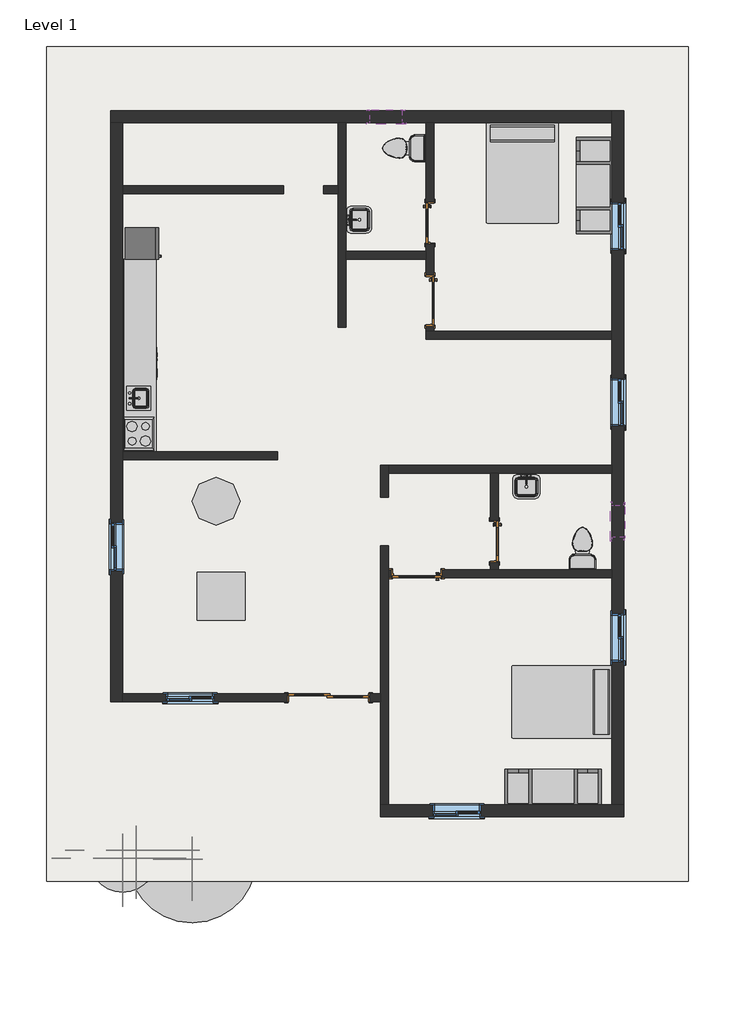
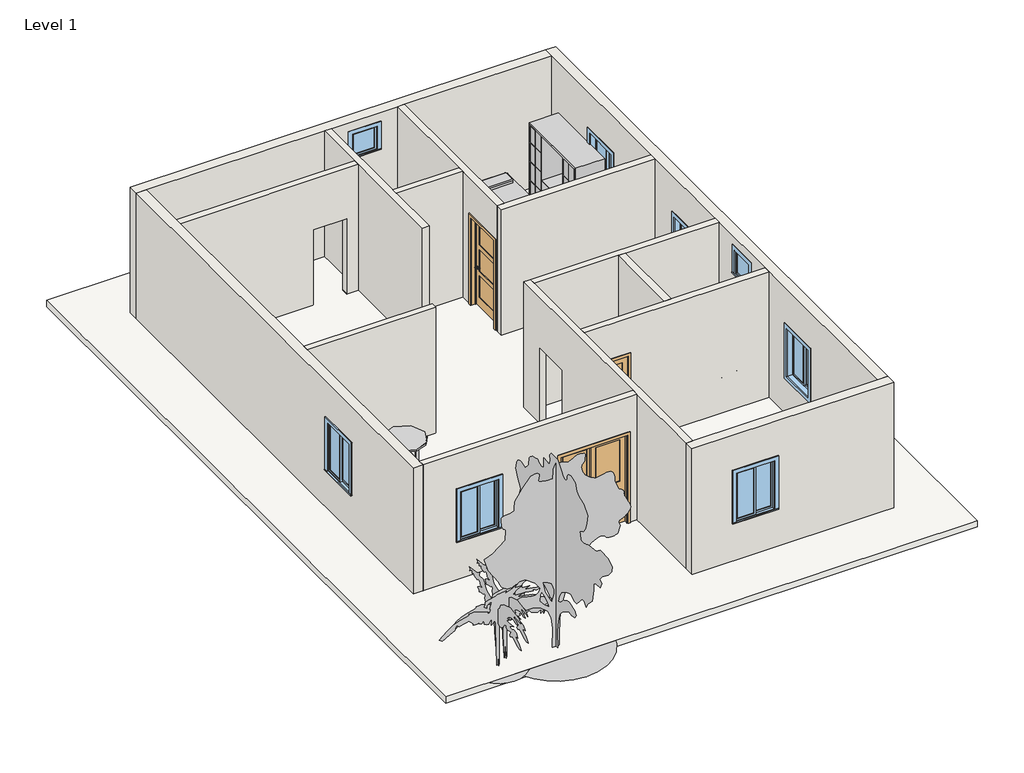
# One storey, incomplete: 15 walls, 8 windows, 7 furniture elements, 5 doors, 5 flow terminals, 4 proxies, 3 geographic elements, 1 slab.
"""IFC4 building model written with IfcOpenShell, lengths in millimetres."""

from ifc_helpers import new_model, si_unit, frame, origin, origin_with_axes, place, context, project, spatial, polyline, outline, extrude, faceted_brep, transform, mapped, element, save
from components import proxy_a6faaae8, proxy_45b28599, kitchenette_medium_kitchenette_medium_2_844211aa, proxy_c523a7b7, door_80d3ddc5, door_a1d926d7, door_7bbed545, door_8959c651, flow_terminal_871c2e40, flow_terminal_62a433f7, toilet_domestic_3d_toilet_domestic_3d_f7549cf7, toilet_domestic_3d_toilet_domestic_3d_183bbd19, furniture_0253826f, furniture_1317d646, furniture_cf0b6580, furniture_905aceb5, furniture_4d44e21c, rpc_tree_deciduous_japanese_cherry_15_e499737d, rpc_tree_tropical_australian_tree_furn_6_77f1a640, window_e25db5b6, window_99c3d43f, window_3ed046d9

model = new_model("IFC4")

# Units and contexts
model_context = context("Model", 3, world=origin())
ifc_project = project(units=[si_unit("LENGTHUNIT", "METRE", prefix="MILLI")], contexts=[model_context])

# Site, building, storey
site = spatial("IfcSite", under=ifc_project)
building = spatial("IfcBuilding", under=site)
storey = spatial("IfcBuildingStorey", under=building, Name="Level 1", Elevation=0.0)

# Proxies
placement = place(None, origin())
proxy_shape = proxy_a6faaae8(model_context)
element("IfcBuildingElementProxy", 1, Name="Cook Top-4 Unit2 : 22\" x 20\"", ObjectType="Cook Top-4 Unit2 : 22\" x 20\"", at=placement, inside=storey, context=model_context, shape_type="MappedRepresentation", body=[
    mapped(proxy_shape, transform((-13786.8447707, 5135.0679528, 0.0), x_axis=(0.0, 1.0000000000000002, 0.0), y_axis=(-1.0000000000000002, 0.0, 0.0), z_axis=(0.0, 0.0, 1.0))),
])
proxy_2_shape = proxy_45b28599(model_context)
element("IfcBuildingElementProxy", 2, Name="Dishwasher : 24\" x 24\" x 34\"", ObjectType="Dishwasher : 24\" x 24\" x 34\"", at=placement, inside=storey, context=model_context, shape_type="MappedRepresentation", body=[
    mapped(proxy_2_shape, transform((-13494.995206, 6086.2504843, 0.0), x_axis=(0.0, 1.0000000000000002, 0.0), y_axis=(-1.0000000000000002, 0.0, 0.0), z_axis=(0.0, 0.0, 1.0))),
])
kitchenette_medium_kitchenette_medium_2_shape = kitchenette_medium_kitchenette_medium_2_844211aa(model_context)
element("IfcBuildingElementProxy", 3, Name="Kitchenette - Medium : Kitchenette - Medium 2", ObjectType="Kitchenette - Medium : Kitchenette - Medium 2", at=placement, inside=storey, context=model_context, shape_type="MappedRepresentation", body=[
    mapped(kitchenette_medium_kitchenette_medium_2_shape, transform((-14091.6447707, 5459.2302479, 0.0), x_axis=(0.0, 1.0000000000000002, 0.0), y_axis=(-1.0000000000000002, 0.0, 0.0), z_axis=(0.0, 0.0, 1.0))),
])
proxy_3_shape = proxy_c523a7b7(model_context)
element("IfcBuildingElementProxy", 4, Name="Refrigerator : 24\" x 25\" LH", ObjectType="Refrigerator : 24\" x 25\" LH", at=placement, inside=storey, context=model_context, shape_type="MappedRepresentation", body=[
    mapped(proxy_3_shape, transform((-13741.1957993, 8748.2179528, 0.0), x_axis=(0.0, 1.0000000000000002, 0.0), y_axis=(-1.0000000000000002, 0.0, 0.0), z_axis=(0.0, 0.0, 1.0))),
])

# Doors
door_shape = door_80d3ddc5(model_context)
element("IfcDoor", 5, ObjectType="Door-Interior-Double-Sliding-2_Panel-Wood : 60\" x 84\"", at=placement, inside=storey, context=model_context, shape_type="MappedRepresentation", body=[
    mapped(door_shape, transform((-10180.0447707, 121.7429528, 0.0), x_axis=(1.0, 0.0, 0.0), y_axis=(0.0, 1.0, 0.0), z_axis=(0.0, 0.0, 1.0))),
])
door_2_shape = door_a1d926d7(model_context)
element("IfcDoor", 6, ObjectType="Door-Interior-Single-1_Panel-Wood : 30\" x 80\"", at=placement, inside=storey, context=model_context, shape_type="MappedRepresentation", body=[
    mapped(door_2_shape, transform((-7027.2697707, 3090.3679528, 0.0), x_axis=(0.0, -1.0, 0.0), y_axis=(1.0, 0.0, 0.0), z_axis=(0.0, 0.0, 1.0))),
])
door_3_shape = door_7bbed545(model_context)
element("IfcDoor", 7, ObjectType="Door-Interior-Single-1_Panel-Wood : 30\" x 80\"", at=placement, inside=storey, context=model_context, shape_type="MappedRepresentation", body=[
    mapped(door_3_shape, transform((-8252.8197707, 9135.5679528, 0.0), x_axis=(0.0, -1.0, 0.0), y_axis=(1.0, 0.0, 0.0), z_axis=(0.0, 0.0, 1.0))),
])
door_4_shape = door_8959c651(model_context)
element("IfcDoor", 8, ObjectType="Door-Interior-Single-3_Panel_Vert-Wood : 36\" x 84\"", at=placement, inside=storey, context=model_context, shape_type="MappedRepresentation", body=[
    mapped(door_4_shape, transform((-8503.6447707, 2477.5929528, 0.0), x_axis=(-1.0, 0.0, 0.0), y_axis=(0.0, -1.0, 0.0), z_axis=(0.0, 0.0, 1.0))),
])
element("IfcDoor", 9, ObjectType="Door-Interior-Single-3_Panel_Vert-Wood : 36\" x 84\"", at=placement, inside=storey, context=model_context, shape_type="MappedRepresentation", body=[
    mapped(door_4_shape, transform((-8246.4697707, 7662.3679528, 0.0), x_axis=(0.0, -1.0, 0.0), y_axis=(1.0, 0.0, 0.0), z_axis=(0.0, 0.0, 1.0))),
])

# Flow terminals
flow_terminal_shape = flow_terminal_871c2e40(model_context)
element("IfcFlowTerminal", 10, ObjectType="Sink Kitchen-Island : 18\" x 18\"", at=placement, inside=storey, context=model_context, shape_type="MappedRepresentation", body=[
    mapped(flow_terminal_shape, transform((-13784.4993696, 5792.4787122, -14.4), x_axis=(0.0, 1.0000000000000002, 0.0), y_axis=(-1.0000000000000002, 0.0, 0.0), z_axis=(0.0, 0.0, 1.0))),
])
flow_terminal_2_shape = flow_terminal_62a433f7(model_context)
element("IfcFlowTerminal", 11, ObjectType="Sink Vanity-Square : 20\" x 18\"", at=placement, inside=storey, context=model_context, shape_type="MappedRepresentation", body=[
    mapped(flow_terminal_2_shape, transform((-9644.2993696, 9183.3787122, 0.0), x_axis=(0.0, 1.0000000000000002, 0.0), y_axis=(-1.0000000000000002, 0.0, 0.0), z_axis=(0.0, 0.0, 1.0))),
])
element("IfcFlowTerminal", 12, ObjectType="Sink Vanity-Square : 20\" x 18\"", at=placement, inside=storey, context=model_context, shape_type="MappedRepresentation", body=[
    mapped(flow_terminal_2_shape, transform((-6436.5340113, 4180.2225517, 0.0), x_axis=(1.0000000000000007, 0.0, 0.0), y_axis=(0.0, 1.0000000000000007, 0.0), z_axis=(0.0, 0.0, 1.0))),
])
toilet_domestic_3d_toilet_domestic_3d_shape = toilet_domestic_3d_toilet_domestic_3d_f7549cf7(model_context)
toilet_domestic_3d_toilet_domestic_3d_2_shape = toilet_domestic_3d_toilet_domestic_3d_183bbd19(model_context)
element("IfcFlowTerminal", 13, ObjectType="Toilet-Domestic-3D : Toilet-Domestic-3D", at=placement, inside=storey, context=model_context, shape_type="MappedRepresentation", body=[
    mapped(toilet_domestic_3d_toilet_domestic_3d_shape, transform((-8845.9407981, 10557.9679528, 0.0), x_axis=(0.0, -1.0000000000000004, 0.0), y_axis=(1.0000000000000004, 0.0, 0.0), z_axis=(0.0, 0.0, 1.0))),
    mapped(toilet_domestic_3d_toilet_domestic_3d_2_shape, transform((-8845.9407981, 10557.9679528, 0.0), x_axis=(0.0, -1.0000000000000004, 0.0), y_axis=(1.0000000000000004, 0.0, 0.0), z_axis=(0.0, 0.0, 1.0))),
])
element("IfcFlowTerminal", 14, ObjectType="Toilet-Domestic-3D : Toilet-Domestic-3D", at=placement, inside=storey, context=model_context, shape_type="MappedRepresentation", body=[
    mapped(toilet_domestic_3d_toilet_domestic_3d_shape, transform((-5354.0447707, 3051.6639802, 0.0), x_axis=(-1.0000000000000004, 0.0, 0.0), y_axis=(0.0, -1.0000000000000004, 0.0), z_axis=(0.0, 0.0, 1.0))),
    mapped(toilet_domestic_3d_toilet_domestic_3d_2_shape, transform((-5354.0447707, 3051.6639802, 0.0), x_axis=(-1.0000000000000004, 0.0, 0.0), y_axis=(0.0, -1.0000000000000004, 0.0), z_axis=(0.0, 0.0, 1.0))),
])

# Furniture
furniture_shape = furniture_0253826f(model_context)
element("IfcFurniture", 15, ObjectType="Bed-Standard : Double 54\" x 75\"", at=placement, inside=storey, context=model_context, shape_type="MappedRepresentation", body=[
    mapped(furniture_shape, transform((-6768.5332953, 10133.6630348, 0.0), x_axis=(1.0, 0.0, 0.0), y_axis=(0.0, 1.0, 0.0), z_axis=(0.0, 0.0, 1.0))),
])
element("IfcFurniture", 16, ObjectType="Bed-Standard : Double 54\" x 75\"", at=placement, inside=storey, context=model_context, shape_type="MappedRepresentation", body=[
    mapped(furniture_shape, transform((-5702.1496888, 313.8564774, 0.0), x_axis=(0.0, -1.0, 0.0), y_axis=(1.0, 0.0, 0.0), z_axis=(0.0, 0.0, 1.0))),
])
furniture_2_shape = furniture_1317d646(model_context)
element("IfcFurniture", 17, ObjectType="Counter Top w Sink Hole : 24\" Depth", at=placement, inside=storey, context=model_context, shape_type="MappedRepresentation", body=[
    mapped(furniture_2_shape, transform((-14091.6447707, 5992.6302479, -14.4), x_axis=(0.0, 1.0000000000000002, 0.0), y_axis=(-1.0000000000000002, 0.0, 0.0), z_axis=(0.0, 0.0, 1.0))),
])
furniture_3_shape = furniture_cf0b6580(model_context)
element("IfcFurniture", 18, ObjectType="Entertainment Center : 72\" x 72\" x 24\"", at=placement, inside=storey, context=model_context, shape_type="MappedRepresentation", body=[
    mapped(furniture_3_shape, transform((-5912.8447707, -2015.0320472, 0.0), x_axis=(-1.0, 0.0, 0.0), y_axis=(0.0, -1.0, 0.0), z_axis=(0.0, 0.0, 1.0))),
])
element("IfcFurniture", 19, ObjectType="Entertainment Center : 72\" x 72\" x 24\"", at=placement, inside=storey, context=model_context, shape_type="MappedRepresentation", body=[
    mapped(furniture_3_shape, transform((-4693.6447707, 9846.7679528, 0.0), x_axis=(0.0, -1.0000000000000002, 0.0), y_axis=(1.0000000000000002, 0.0, 0.0), z_axis=(0.0, 0.0, 1.0))),
])
furniture_4_shape = furniture_905aceb5(model_context)
element("IfcFurniture", 20, ObjectType="Table-Dining Round w Chairs : 36\" Diameter", at=placement, inside=storey, context=model_context, shape_type="MappedRepresentation", body=[
    mapped(furniture_4_shape, transform((-12417.326738, 4037.2466413, 0.0), x_axis=(1.0, 0.0, 0.0), y_axis=(0.0, 1.0, 0.0), z_axis=(0.0, 0.0, 1.0))),
])
furniture_5_shape = furniture_4d44e21c(model_context)
element("IfcFurniture", 21, ObjectType="Table-Rectangular : 36\" x 36\"", at=placement, inside=storey, context=model_context, shape_type="MappedRepresentation", body=[
    mapped(furniture_5_shape, transform((-12224.7447707, 2048.9679528, 0.0), x_axis=(0.0, 1.0000000000000002, 0.0), y_axis=(-1.0000000000000002, 0.0, 0.0), z_axis=(0.0, 0.0, 1.0))),
])

# Geographic elements
rpc_tree_deciduous_japanese_cherry_15_shape = rpc_tree_deciduous_japanese_cherry_15_e499737d(model_context)
element("IfcGeographicElement", 22, ObjectType="RPC Tree - Deciduous : Japanese Cherry - 15'", at=placement, inside=storey, context=model_context, shape_type="MappedRepresentation", body=[
    mapped(rpc_tree_deciduous_japanese_cherry_15_shape, transform((-12770.8447707, -2942.1320472, 0.0), x_axis=(1.0, 0.0, 0.0), y_axis=(0.0, 1.0, 0.0), z_axis=(0.0, 0.0, 1.0))),
])
rpc_tree_tropical_australian_tree_furn_6_shape = rpc_tree_tropical_australian_tree_furn_6_77f1a640(model_context)
element("IfcGeographicElement", 23, ObjectType="RPC Tree - Tropical : Australian Tree Furn - 6'", at=placement, inside=storey, context=model_context, shape_type="MappedRepresentation", body=[
    mapped(rpc_tree_tropical_australian_tree_furn_6_shape, transform((-13837.6447707, -2777.0320472, 0.0), x_axis=(1.0, 0.0, 0.0), y_axis=(0.0, 1.0, 0.0), z_axis=(0.0, 0.0, 1.0))),
])
element("IfcGeographicElement", 24, ObjectType="RPC Tree - Tropical : Australian Tree Furn - 6'", at=placement, inside=storey, context=model_context, shape_type="MappedRepresentation", body=[
    mapped(rpc_tree_tropical_australian_tree_furn_6_shape, transform((-14091.6447707, -2929.4320472, 0.0), x_axis=(1.0, 0.0, 0.0), y_axis=(0.0, 1.0, 0.0), z_axis=(0.0, 0.0, 1.0))),
])

# Slab
element("IfcSlab", 25, ObjectType="Generic - 6\" 2", at=placement, inside=storey, context=model_context, shape_type="SweptSolid", body=[
    extrude(outline(polyline([(-3347.4447707, 12488.3679528), (-3347.4447707, -3361.2320472), (-15539.4447707, -3361.2320472), (-15539.4447707, 12488.3679528), (-3347.4447707, 12488.3679528)])), frame((0.0, 0.0, -152.4), z_axis=(0.0, 0.0, 1.0), x_axis=(1.0, 0.0, 0.0)), (0.0, 0.0, 1.0), 152.4),
])

# Walls
element("IfcWall", 26, ObjectType="Generic - 6\"", at=placement, inside=storey, context=model_context, shape_type="Brep", body=[
    faceted_brep([(-4795.2447707, 7078.1679528, 0.0), (-8173.4447707, 7078.1679528, 0.0), (-8325.8447707, 7078.1679528, 0.0), (-8325.8447707, 7078.1679528, 3048.0), (-8173.4447707, 7078.1679528, 3048.0), (-4795.2447707, 7078.1679528, 3048.0), (-4795.2447707, 6925.7679528, 0.0), (-4795.2447707, 6925.7679528, 3048.0), (-8325.8447707, 6925.7679528, 3048.0), (-8325.8447707, 6925.7679528, 0.0)], [[[0, 1, 2, 3, 4, 5]], [[6, 7, 8, 9]], [[2, 1, 0, 6, 9]], [[5, 4, 3, 8, 7]], [[0, 5, 7, 6]], [[3, 2, 9, 8]]]),
])
element("IfcWall", 27, ObjectType="Generic - 6\"", at=placement, inside=storey, context=model_context, shape_type="Brep", body=[
    faceted_brep([(-8325.8447707, 7078.1679528, 3048.0), (-8325.8447707, 8449.7679528, 3048.0), (-8325.8447707, 8602.1679528, 3048.0), (-8325.8447707, 11040.5679528, 3048.0), (-8325.8447707, 11040.5679528, 0.0), (-8325.8447707, 9541.9679528, 0.0), (-8325.8447707, 9541.9679528, 2057.4), (-8325.8447707, 8729.1679528, 2057.4), (-8325.8447707, 8729.1679528, 0.0), (-8325.8447707, 8602.1679528, 0.0), (-8325.8447707, 8449.7679528, 0.0), (-8325.8447707, 8144.9679528, 0.0), (-8325.8447707, 8144.9679528, 2159.0), (-8325.8447707, 7179.7679528, 2159.0), (-8325.8447707, 7179.7679528, 0.0), (-8325.8447707, 7078.1679528, 0.0), (-8173.4447707, 11040.5679528, 3048.0), (-8173.4447707, 7078.1679528, 3048.0), (-8173.4447707, 7078.1679528, 0.0), (-8173.4447707, 7179.7679528, 0.0), (-8173.4447707, 7179.7679528, 2159.0), (-8173.4447707, 8144.9679528, 2159.0), (-8173.4447707, 8144.9679528, 0.0), (-8173.4447707, 8729.1679528, 0.0), (-8173.4447707, 8729.1679528, 2057.4), (-8173.4447707, 9541.9679528, 2057.4), (-8173.4447707, 9541.9679528, 0.0), (-8173.4447707, 11040.5679528, 0.0)], [[[0, 1, 2, 3, 4, 5, 6, 7, 8, 9, 10, 11, 12, 13, 14, 15]], [[16, 17, 18, 19, 20, 21, 22, 23, 24, 25, 26, 27]], [[4, 27, 26, 5]], [[18, 15, 14, 19]], [[22, 11, 10, 9, 8, 23]], [[3, 2, 1, 0, 17, 16]], [[4, 3, 16, 27]], [[0, 15, 18, 17]], [[13, 20, 19, 14]], [[20, 13, 12, 21]], [[21, 12, 11, 22]], [[7, 24, 23, 8]], [[24, 7, 6, 25]], [[25, 6, 5, 26]]]),
])
element("IfcWall", 28, ObjectType="Generic - 6\"", at=placement, inside=storey, context=model_context, shape_type="SweptSolid", body=[
    extrude(outline(polyline([(-9849.8447707, 8602.1679528), (-8325.8447707, 8602.1679528), (-8325.8447707, 8449.7679528), (-9849.8447707, 8449.7679528), (-9849.8447707, 8602.1679528)])), origin_with_axes(), (0.0, 0.0, 1.0), 3048.0),
])
element("IfcWall", 29, ObjectType="Generic - 6\"", at=placement, inside=storey, context=model_context, shape_type="Brep", body=[
    faceted_brep([(-10002.2447707, 11040.5679528, 0.0), (-10002.2447707, 9846.7679528, 0.0), (-10002.2447707, 9694.3679528, 0.0), (-10002.2447707, 7154.3679528, 0.0), (-10002.2447707, 7154.3679528, 3048.0), (-10002.2447707, 9694.3679528, 3048.0), (-10002.2447707, 9846.7679528, 3048.0), (-10002.2447707, 11040.5679528, 3048.0), (-9849.8447707, 11040.5679528, 0.0), (-9849.8447707, 11040.5679528, 3048.0), (-9849.8447707, 8602.1679528, 3048.0), (-9849.8447707, 8449.7679528, 3048.0), (-9849.8447707, 7154.3679528, 3048.0), (-9849.8447707, 7154.3679528, 0.0), (-9849.8447707, 8449.7679528, 0.0), (-9849.8447707, 8602.1679528, 0.0)], [[[0, 1, 2, 3, 4, 5, 6, 7]], [[8, 9, 10, 11, 12, 13, 14, 15]], [[3, 2, 1, 0, 8, 15, 14, 13]], [[4, 3, 13, 12]], [[7, 6, 5, 4, 12, 11, 10, 9]], [[0, 7, 9, 8]]]),
])
element("IfcWall", 30, ObjectType="Generic - 6\"", at=placement, inside=storey, context=model_context, shape_type="SweptSolid", body=[
    extrude(outline(polyline([(0.0, -10002.2447707), (3048.0, -10002.2447707), (3048.0, -14091.6447707), (0.0, -14091.6447707), (0.0, -11037.2947707), (12.7, -11037.2947707), (1828.8, -11037.2947707), (1828.8, -10275.2947707), (12.7, -10275.2947707), (0.0, -10275.2947707), (0.0, -10002.2447707)])), frame((0.0, 9694.3679528, 0.0), z_axis=(0.0, 1.0, 0.0), x_axis=(0.0, 0.0, 1.0)), (0.0, 0.0, 1.0), 152.4),
])
element("IfcWall", 31, ObjectType="Generic - 6\"", at=placement, inside=storey, context=model_context, shape_type="SweptSolid", body=[
    extrude(outline(polyline([(3048.0, -9189.4447707), (3048.0, -14091.6447707), (0.0, -14091.6447707), (0.0, -10967.4447707), (2159.0, -10967.4447707), (2159.0, -9392.6447707), (0.0, -9392.6447707), (0.0, -9189.4447707), (3048.0, -9189.4447707)]), holes=[polyline([(2133.6, -13266.1447707), (2133.6, -12351.7447707), (914.4, -12351.7447707), (914.4, -13266.1447707), (2133.6, -13266.1447707)])]), frame((0.0, 42.3679528, 0.0), z_axis=(0.0, 1.0, 0.0), x_axis=(0.0, 0.0, 1.0)), (0.0, 0.0, 1.0), 152.4),
])
element("IfcWall", 32, ObjectType="Generic - 6\"", at=placement, inside=storey, context=model_context, shape_type="Brep", body=[
    faceted_brep([(-9189.4447707, 4538.1679528, 0.0), (-9189.4447707, 3925.3929528, 0.0), (-9189.4447707, 3925.3929528, 1828.8), (-9189.4447707, 3010.9929528, 1828.8), (-9189.4447707, 3010.9929528, 0.0), (-9189.4447707, 194.7679528, 0.0), (-9189.4447707, 42.3679528, 0.0), (-9189.4447707, -1913.4320472, 0.0), (-9189.4447707, -1913.4320472, 3048.0), (-9189.4447707, 42.3679528, 3048.0), (-9189.4447707, 194.7679528, 3048.0), (-9189.4447707, 4538.1679528, 3048.0), (-9037.0447707, 4538.1679528, 0.0), (-9037.0447707, 4538.1679528, 3048.0), (-9037.0447707, 4385.7679528, 3048.0), (-9037.0447707, 2556.9679528, 3048.0), (-9037.0447707, 2404.5679528, 3048.0), (-9037.0447707, -1913.4320472, 3048.0), (-9037.0447707, -1913.4320472, 0.0), (-9037.0447707, 2404.5679528, 0.0), (-9037.0447707, 2556.9679528, 0.0), (-9037.0447707, 3010.9929528, 0.0), (-9037.0447707, 3010.9929528, 1828.8), (-9037.0447707, 3925.3929528, 1828.8), (-9037.0447707, 3925.3929528, 0.0), (-9037.0447707, 4385.7679528, 0.0)], [[[0, 1, 2, 3, 4, 5, 6, 7, 8, 9, 10, 11]], [[12, 13, 14, 15, 16, 17, 18, 19, 20, 21, 22, 23, 24, 25]], [[0, 11, 13, 12]], [[8, 7, 18, 17]], [[1, 0, 12, 25, 24]], [[11, 10, 9, 8, 17, 16, 15, 14, 13]], [[2, 1, 24, 23]], [[3, 2, 23, 22]], [[4, 3, 22, 21]], [[7, 6, 5, 4, 21, 20, 19, 18]]]),
])
element("IfcWall", 33, ObjectType="Generic - 6\"", at=placement, inside=storey, context=model_context, shape_type="Brep", body=[
    faceted_brep([(-9037.0447707, 2556.9679528, 3048.0), (-7106.6447707, 2556.9679528, 3048.0), (-6954.2447707, 2556.9679528, 3048.0), (-4795.2447707, 2556.9679528, 3048.0), (-4795.2447707, 2556.9679528, 0.0), (-6954.2447707, 2556.9679528, 0.0), (-7106.6447707, 2556.9679528, 0.0), (-8021.0447707, 2556.9679528, 0.0), (-8021.0447707, 2556.9679528, 2159.0), (-8986.2447707, 2556.9679528, 2159.0), (-8986.2447707, 2556.9679528, 0.0), (-9037.0447707, 2556.9679528, 0.0), (-4795.2447707, 2404.5679528, 3048.0), (-9037.0447707, 2404.5679528, 3048.0), (-9037.0447707, 2404.5679528, 0.0), (-8986.2447707, 2404.5679528, 0.0), (-8986.2447707, 2404.5679528, 2159.0), (-8021.0447707, 2404.5679528, 2159.0), (-8021.0447707, 2404.5679528, 0.0), (-4795.2447707, 2404.5679528, 0.0)], [[[0, 1, 2, 3, 4, 5, 6, 7, 8, 9, 10, 11]], [[12, 13, 14, 15, 16, 17, 18, 19]], [[4, 19, 18, 7, 6, 5]], [[14, 11, 10, 15]], [[3, 2, 1, 0, 13, 12]], [[4, 3, 12, 19]], [[0, 11, 14, 13]], [[9, 16, 15, 10]], [[16, 9, 8, 17]], [[17, 8, 7, 18]]]),
])
element("IfcWall", 34, ObjectType="Generic - 6\"", at=placement, inside=storey, context=model_context, shape_type="Brep", body=[
    faceted_brep([(-4795.2447707, 4538.1679528, 0.0), (-9037.0447707, 4538.1679528, 0.0), (-9037.0447707, 4538.1679528, 3048.0), (-4795.2447707, 4538.1679528, 3048.0), (-4795.2447707, 4385.7679528, 0.0), (-4795.2447707, 4385.7679528, 3048.0), (-6954.2447707, 4385.7679528, 3048.0), (-7106.6447707, 4385.7679528, 3048.0), (-9037.0447707, 4385.7679528, 3048.0), (-9037.0447707, 4385.7679528, 0.0), (-7106.6447707, 4385.7679528, 0.0), (-6954.2447707, 4385.7679528, 0.0)], [[[0, 1, 2, 3]], [[4, 5, 6, 7, 8, 9, 10, 11]], [[1, 0, 4, 11, 10, 9]], [[3, 2, 8, 7, 6, 5]], [[0, 3, 5, 4]], [[2, 1, 9, 8]]]),
])
element("IfcWall", 35, ObjectType="Generic - 6\"", at=placement, inside=storey, context=model_context, shape_type="SweptSolid", body=[
    extrude(outline(polyline([(2556.9679528, 3048.0), (4385.7679528, 3048.0), (4385.7679528, 0.0), (3496.7679528, 0.0), (3496.7679528, 2057.4), (2683.9679528, 2057.4), (2683.9679528, 0.0), (2556.9679528, 0.0), (2556.9679528, 3048.0)])), frame((-7106.6447707, 0.0, 0.0), z_axis=(1.0, 0.0, 0.0), x_axis=(0.0, 1.0, 0.0)), (0.0, 0.0, 1.0), 152.4),
])
element("IfcWall", 36, ObjectType="Generic - 6\"", at=placement, inside=storey, context=model_context, shape_type="SweptSolid", body=[
    extrude(outline(polyline([(-14091.6447707, 4792.1679528), (-11145.2447707, 4792.1679528), (-11145.2447707, 4639.7679528), (-14091.6447707, 4639.7679528), (-14091.6447707, 4792.1679528)])), origin_with_axes(), (0.0, 0.0, 1.0), 3048.0),
])
element("IfcWall", 37, ObjectType="Generic - 9\" 2", at=placement, inside=storey, context=model_context, shape_type="Brep", body=[
    faceted_brep([(-14320.2447707, 11040.5679528, 0.0), (-14091.6447707, 11040.5679528, 0.0), (-10002.2447707, 11040.5679528, 0.0), (-9849.8447707, 11040.5679528, 0.0), (-8325.8447707, 11040.5679528, 0.0), (-8173.4447707, 11040.5679528, 0.0), (-4795.2447707, 11040.5679528, 0.0), (-4795.2447707, 11040.5679528, 3048.0), (-8173.4447707, 11040.5679528, 3048.0), (-8325.8447707, 11040.5679528, 3048.0), (-9849.8447707, 11040.5679528, 3048.0), (-10002.2447707, 11040.5679528, 3048.0), (-14091.6447707, 11040.5679528, 3048.0), (-14320.2447707, 11040.5679528, 3048.0), (-9392.6447707, 11040.5679528, 2768.6), (-8783.0447707, 11040.5679528, 2768.6), (-8783.0447707, 11040.5679528, 2159.0), (-9392.6447707, 11040.5679528, 2159.0), (-14320.2447707, 11269.1679528, 0.0), (-14320.2447707, 11269.1679528, 3048.0), (-4795.2447707, 11269.1679528, 3048.0), (-4795.2447707, 11269.1679528, 0.0), (-9392.6447707, 11269.1679528, 2768.6), (-9392.6447707, 11269.1679528, 2159.0), (-8783.0447707, 11269.1679528, 2159.0), (-8783.0447707, 11269.1679528, 2768.6)], [[[0, 1, 2, 3, 4, 5, 6, 7, 8, 9, 10, 11, 12, 13], [14, 15, 16, 17]], [[18, 19, 20, 21], [22, 23, 24, 25]], [[6, 5, 4, 3, 2, 1, 0, 18, 21]], [[13, 12, 11, 10, 9, 8, 7, 20, 19]], [[0, 13, 19, 18]], [[7, 6, 21, 20]], [[23, 22, 14, 17]], [[24, 23, 17, 16]], [[25, 24, 16, 15]], [[22, 25, 15, 14]]]),
])
element("IfcWall", 38, ObjectType="Generic - 9\" 2", at=placement, inside=storey, context=model_context, shape_type="Brep", body=[
    faceted_brep([(-14091.6447707, 42.3679528, 0.0), (-14091.6447707, 194.7679528, 0.0), (-14091.6447707, 4639.7679528, 0.0), (-14091.6447707, 4792.1679528, 0.0), (-14091.6447707, 9694.3679528, 0.0), (-14091.6447707, 9846.7679528, 0.0), (-14091.6447707, 11040.5679528, 0.0), (-14091.6447707, 11040.5679528, 3048.0), (-14091.6447707, 9846.7679528, 3048.0), (-14091.6447707, 9694.3679528, 3048.0), (-14091.6447707, 4792.1679528, 3048.0), (-14091.6447707, 4639.7679528, 3048.0), (-14091.6447707, 194.7679528, 3048.0), (-14091.6447707, 42.3679528, 3048.0), (-14091.6447707, 3445.9679528, 2133.6), (-14091.6447707, 3445.9679528, 914.4), (-14091.6447707, 2531.5679528, 914.4), (-14091.6447707, 2531.5679528, 2133.6), (-14320.2447707, 42.3679528, 0.0), (-14320.2447707, 42.3679528, 3048.0), (-14320.2447707, 11040.5679528, 3048.0), (-14320.2447707, 11040.5679528, 0.0), (-14320.2447707, 3445.9679528, 2133.6), (-14320.2447707, 2531.5679528, 2133.6), (-14320.2447707, 2531.5679528, 914.4), (-14320.2447707, 3445.9679528, 914.4)], [[[0, 1, 2, 3, 4, 5, 6, 7, 8, 9, 10, 11, 12, 13], [14, 15, 16, 17]], [[18, 19, 20, 21], [22, 23, 24, 25]], [[6, 5, 4, 3, 2, 1, 0, 18, 21]], [[13, 12, 11, 10, 9, 8, 7, 20, 19]], [[7, 6, 21, 20]], [[15, 14, 22, 25]], [[16, 15, 25, 24]], [[17, 16, 24, 23]], [[14, 17, 23, 22]], [[0, 13, 19, 18]]]),
])
element("IfcWall", 39, ObjectType="Generic - 9\" 2", at=placement, inside=storey, context=model_context, shape_type="Brep", body=[
    faceted_brep([(-4566.6447707, -1913.4320472, 0.0), (-4795.2447707, -1913.4320472, 0.0), (-9037.0447707, -1913.4320472, 0.0), (-9189.4447707, -1913.4320472, 0.0), (-9189.4447707, -1913.4320472, 3048.0), (-9037.0447707, -1913.4320472, 3048.0), (-4795.2447707, -1913.4320472, 3048.0), (-4566.6447707, -1913.4320472, 3048.0), (-8198.8447707, -1913.4320472, 2133.6), (-8198.8447707, -1913.4320472, 914.4), (-7284.4447707, -1913.4320472, 914.4), (-7284.4447707, -1913.4320472, 2133.6), (-4566.6447707, -2142.0320472, 0.0), (-4566.6447707, -2142.0320472, 3048.0), (-9189.4447707, -2142.0320472, 3048.0), (-9189.4447707, -2142.0320472, 0.0), (-8198.8447707, -2142.0320472, 2133.6), (-7284.4447707, -2142.0320472, 2133.6), (-7284.4447707, -2142.0320472, 914.4), (-8198.8447707, -2142.0320472, 914.4)], [[[0, 1, 2, 3, 4, 5, 6, 7], [8, 9, 10, 11]], [[12, 13, 14, 15], [16, 17, 18, 19]], [[3, 2, 1, 0, 12, 15]], [[7, 6, 5, 4, 14, 13]], [[0, 7, 13, 12]], [[4, 3, 15, 14]], [[9, 8, 16, 19]], [[10, 9, 19, 18]], [[11, 10, 18, 17]], [[8, 11, 17, 16]]]),
])
element("IfcWall", 40, ObjectType="Generic - 9\" 2", at=placement, inside=storey, context=model_context, shape_type="Brep", body=[
    faceted_brep([(-4795.2447707, 11269.1679528, 0.0), (-4795.2447707, 11040.5679528, 0.0), (-4795.2447707, 7078.1679528, 0.0), (-4795.2447707, 6925.7679528, 0.0), (-4795.2447707, 4538.1679528, 0.0), (-4795.2447707, 4385.7679528, 0.0), (-4795.2447707, 2556.9679528, 0.0), (-4795.2447707, 2404.5679528, 0.0), (-4795.2447707, -1913.4320472, 0.0), (-4795.2447707, -1913.4320472, 3048.0), (-4795.2447707, 2404.5679528, 3048.0), (-4795.2447707, 2556.9679528, 3048.0), (-4795.2447707, 4385.7679528, 3048.0), (-4795.2447707, 4538.1679528, 3048.0), (-4795.2447707, 6925.7679528, 3048.0), (-4795.2447707, 7078.1679528, 3048.0), (-4795.2447707, 11040.5679528, 3048.0), (-4795.2447707, 11269.1679528, 3048.0), (-4795.2447707, 5274.7679528, 2133.6), (-4795.2447707, 5274.7679528, 914.4), (-4795.2447707, 6189.1679528, 914.4), (-4795.2447707, 6189.1679528, 2133.6), (-4795.2447707, 8621.2179528, 2133.6), (-4795.2447707, 8621.2179528, 914.4), (-4795.2447707, 9535.6179528, 914.4), (-4795.2447707, 9535.6179528, 2133.6), (-4795.2447707, 804.3679528, 2133.6), (-4795.2447707, 804.3679528, 914.4), (-4795.2447707, 1718.7679528, 914.4), (-4795.2447707, 1718.7679528, 2133.6), (-4795.2447707, 3776.1679528, 2768.6), (-4795.2447707, 3166.5679528, 2768.6), (-4795.2447707, 3166.5679528, 2159.0), (-4795.2447707, 3776.1679528, 2159.0), (-4566.6447707, 11269.1679528, 0.0), (-4566.6447707, 11269.1679528, 3048.0), (-4566.6447707, -1913.4320472, 3048.0), (-4566.6447707, -1913.4320472, 0.0), (-4566.6447707, 5274.7679528, 2133.6), (-4566.6447707, 6189.1679528, 2133.6), (-4566.6447707, 6189.1679528, 914.4), (-4566.6447707, 5274.7679528, 914.4), (-4566.6447707, 8621.2179528, 2133.6), (-4566.6447707, 9535.6179528, 2133.6), (-4566.6447707, 9535.6179528, 914.4), (-4566.6447707, 8621.2179528, 914.4), (-4566.6447707, 804.3679528, 2133.6), (-4566.6447707, 1718.7679528, 2133.6), (-4566.6447707, 1718.7679528, 914.4), (-4566.6447707, 804.3679528, 914.4), (-4566.6447707, 3776.1679528, 2768.6), (-4566.6447707, 3776.1679528, 2159.0), (-4566.6447707, 3166.5679528, 2159.0), (-4566.6447707, 3166.5679528, 2768.6)], [[[0, 1, 2, 3, 4, 5, 6, 7, 8, 9, 10, 11, 12, 13, 14, 15, 16, 17], [18, 19, 20, 21], [22, 23, 24, 25], [26, 27, 28, 29], [30, 31, 32, 33]], [[34, 35, 36, 37], [38, 39, 40, 41], [42, 43, 44, 45], [46, 47, 48, 49], [50, 51, 52, 53]], [[8, 7, 6, 5, 4, 3, 2, 1, 0, 34, 37]], [[17, 16, 15, 14, 13, 12, 11, 10, 9, 36, 35]], [[0, 17, 35, 34]], [[9, 8, 37, 36]], [[19, 18, 38, 41]], [[20, 19, 41, 40]], [[21, 20, 40, 39]], [[18, 21, 39, 38]], [[23, 22, 42, 45]], [[24, 23, 45, 44]], [[25, 24, 44, 43]], [[22, 25, 43, 42]], [[27, 26, 46, 49]], [[28, 27, 49, 48]], [[29, 28, 48, 47]], [[26, 29, 47, 46]], [[51, 50, 30, 33]], [[52, 51, 33, 32]], [[53, 52, 32, 31]], [[50, 53, 31, 30]]]),
])

# Windows
window_shape = window_e25db5b6(model_context)
element("IfcWindow", 41, ObjectType="Slider with Trim : 36\" x 48\"", at=placement, inside=storey, context=model_context, shape_type="MappedRepresentation", body=[
    mapped(window_shape, transform((-14205.9447707, 2988.7679528, 0.0), x_axis=(0.0, 1.0, 0.0), y_axis=(-1.0, 0.0, 0.0), z_axis=(0.0, 0.0, 1.0))),
])
element("IfcWindow", 42, ObjectType="Slider with Trim : 36\" x 48\"", at=placement, inside=storey, context=model_context, shape_type="MappedRepresentation", body=[
    mapped(window_shape, transform((-4680.9447707, 5731.9679528, 0.0), x_axis=(0.0, -1.0, 0.0), y_axis=(1.0, 0.0, 0.0), z_axis=(0.0, 0.0, 1.0))),
])
element("IfcWindow", 43, ObjectType="Slider with Trim : 36\" x 48\"", at=placement, inside=storey, context=model_context, shape_type="MappedRepresentation", body=[
    mapped(window_shape, transform((-4680.9447707, 9078.4179528, 0.0), x_axis=(0.0, -1.0, 0.0), y_axis=(1.0, 0.0, 0.0), z_axis=(0.0, 0.0, 1.0))),
])
element("IfcWindow", 44, ObjectType="Slider with Trim : 36\" x 48\"", at=placement, inside=storey, context=model_context, shape_type="MappedRepresentation", body=[
    mapped(window_shape, transform((-7741.6447707, -2027.7320472, 0.0), x_axis=(-1.0, 0.0, 0.0), y_axis=(0.0, -1.0, 0.0), z_axis=(0.0, 0.0, 1.0))),
])
element("IfcWindow", 45, ObjectType="Slider with Trim : 36\" x 48\"", at=placement, inside=storey, context=model_context, shape_type="MappedRepresentation", body=[
    mapped(window_shape, transform((-4680.9447707, 1261.5679528, 0.0), x_axis=(0.0, -1.0, 0.0), y_axis=(1.0, 0.0, 0.0), z_axis=(0.0, 0.0, 1.0))),
])
window_2_shape = window_99c3d43f(model_context)
element("IfcWindow", 46, ObjectType="Slider with Trim : 36\" x 48\"", at=placement, inside=storey, context=model_context, shape_type="MappedRepresentation", body=[
    mapped(window_2_shape, transform((-12808.9447707, 118.5679528, 0.0), x_axis=(-1.0, 0.0, 0.0), y_axis=(0.0, -1.0, 0.0), z_axis=(0.0, 0.0, 1.0))),
])
window_3_shape = window_3ed046d9(model_context)
element("IfcWindow", 47, ObjectType="Transom with Trim : 24\" x 24\"", at=placement, inside=storey, context=model_context, shape_type="MappedRepresentation", body=[
    mapped(window_3_shape, transform((-4680.9447707, 3509.4679528, 0.0), x_axis=(0.0, 1.0, 0.0), y_axis=(-1.0, 0.0, 0.0), z_axis=(0.0, 0.0, 1.0))),
])
element("IfcWindow", 48, ObjectType="Transom with Trim : 24\" x 24\"", at=placement, inside=storey, context=model_context, shape_type="MappedRepresentation", body=[
    mapped(window_3_shape, transform((-9125.9447707, 11154.8679528, 0.0), x_axis=(-1.0, 0.0, 0.0), y_axis=(0.0, -1.0, 0.0), z_axis=(0.0, 0.0, 1.0))),
])

save(model, "model.ifc")

# Revit data of these elements
# Type "Cook Top-4 Unit2 : 22\" x 20\""
#   Depth = 1' - 8"
#   Width = 1' - 10"
#   Burner Material = Steel, Chrome Plated
#   Cooktop Material = Steel, Polished
#   Default Elevation = 0
#   Assembly Code = ""
# Type "Dishwasher : 24\" x 24\" x 34\""
#   Label = "DW"
#   Assembly Code = "E1090400"
#   Depth = 2' - 0"
#   Height = 2' - 10"
#   Width = 2' - 0"
#   Dishwasher Material = Steel, Paint Finish, Ivory, Glossy
#   Panel Face Material = Plastic, Opaque Black
#   Default Elevation = 0
# Type "Kitchenette - Medium : Kitchenette - Medium 2"
#   Assembly Code = "E1090400"
#   Counter Length = 12' - 0"
#   Cabinet Width = 4' - 6"
#   Cabinet Height = 2' - 10 1/2"
#   Cabinet Depth = 2' - 0"
#   Toe Depth = 0' - 3"
#   Toe Height = 0' - 3 1/2"
#   Cabinet Material = Cabinets
#   Door/Drawer Material = Cabinets
#   Handle Material = Cabinets - Handles
#   Default Elevation = 0
# Type "Refrigerator : 24\" x 25\" LH"
#   Label = "REF."
#   Assembly Code = "E1090400"
#   Depth = 2' - 0 3/4"
#   Handle = 0' - 1 1/2"
#   Height = 5' - 3 1/2"
#   Rear Clearance = 0' - 2"
#   Top Door Height = 1' - 8"
#   Width = 1' - 11 1/2"
#   Material = Steel, Paint Finish, Ivory, Glossy
#   Default Elevation = 0
# Type "Door-Interior-Double-Sliding-2_Panel-Wood : 60\" x 84\""
#   Type Mark = "8"
#   Assembly Code = "C1020300"
#   Analytic Construction = "Wooden"
#   Top Rail = 0' - 4 11/16"
#   Thickness = 0' - 1 3/8"
#   Thermal Resistance (R) = 2.5876 (h·ft²·°F)/BTU
#   Stiles = 0' - 4 3/4"
#   Rough Width = 5' - 2"
#   Rough Height = 7' - 1"
#   Lock Rail = 0' - 7 1/2"
#   Height = 7' - 0"
#   Width = 5' - 0"
#   Heat Transfer Coefficient (U) = 0.3865 BTU/(h·ft²·°F)
#   Bottom Rail = 0' - 9 1/8"
#   Trim Material = Cherry
#   Panel Material = Cherry
#   Frame Material = Cherry
#   Visual Light Transmittance = 0
#   Solar Heat Gain Coefficient = 0
#   Wall Closure = (empty or 0)
#   Function = (empty or 0)
# Type "Door-Interior-Single-1_Panel-Wood : 30\" x 80\""
#   Type Mark = "10"
#   Assembly Code = "C1020300"
#   Analytic Construction = "Wooden"
#   Top Rail = 0' - 4 11/16"
#   Thickness = 0' - 1 3/8"
#   Thermal Resistance (R) = 2.5876 (h·ft²·°F)/BTU
#   Swing Angle [instance default] = 90.00°
#   Stiles = 0' - 4 3/4"
#   Rough Width = 2' - 8"
#   Rough Height = 6' - 9"
#   Height = 6' - 8"
#   Width = 2' - 6"
#   Heat Transfer Coefficient (U) = 0.3865 BTU/(h·ft²·°F)
#   Bottom Rail = 0' - 9 1/8"
#   Trim Material = Cherry
#   Panel Material = Cherry
#   Frame Material = Cherry
#   Door Handle Material = Aluminum
#   Visual Light Transmittance = 0
#   Solar Heat Gain Coefficient = 0
#   Wall Closure = (empty or 0)
#   Function = (empty or 0)
# Type "Door-Interior-Single-3_Panel_Vert-Wood : 36\" x 84\""
#   Type Mark = "9"
#   Assembly Code = "C1020300"
#   Analytic Construction = "Wooden"
#   Top Rail = 0' - 4 11/16"
#   Thickness = 0' - 1 3/8"
#   Thermal Resistance (R) = 2.5876 (h·ft²·°F)/BTU
#   Swing Angle [instance default] = 90.00°
#   Stiles = 0' - 4 3/4"
#   Rough Width = 3' - 2"
#   Rough Height = 7' - 1"
#   Intermediate Rail = 0' - 4 1/2"
#   Height = 7' - 0"
#   Width = 3' - 0"
#   Heat Transfer Coefficient (U) = 0.3865 BTU/(h·ft²·°F)
#   Bottom Rail = 0' - 9 1/8"
#   Trim Material = Cherry
#   Panel Material = Cherry
#   Frame Material = Cherry
#   Door Handle Material = Aluminum
#   Visual Light Transmittance = 0
#   Solar Heat Gain Coefficient = 0
#   Wall Closure = (empty or 0)
#   Function = (empty or 0)
# Type "Sink Kitchen-Island : 18\" x 18\""
#   Assembly Code = "D2010410"
#   Counter Height = 3' - 0"
#   Depth = 1' - 6"
#   Width = 1' - 6"
#   Faucet Material = Steel, Polished
#   Sink Material = Steel, Polished
#   Default Elevation = 0
# Type "Sink Vanity-Square : 20\" x 18\""
#   Assembly Code = "D2010400"
#   Counter Height = 2' - 7"
#   Depth = 1' - 6"
#   Width = 1' - 8"
#   Basin Material = Porcelain, Linen
#   Faucet Material = Steel, Polished
#   Default Elevation = 0
# Type "Toilet-Domestic-3D : Toilet-Domestic-3D"
#   Assembly Code = "D2010110"
#   Toilet - Bowl/Basin Material = Porcelain, Linen
#   Toilet - Seat Material = Laminate, Linen, Matte
#   Default Elevation = 0
# Type "Bed-Standard : Double 54\" x 75\""
#   Assembly Code = "E2020200"
#   Length = 6' - 3"
#   Width = 4' - 6"
#   Leg Material = Steel, Chrome Plated
#   Mattress Material = Textile - Bamboo Weave
#   Default Elevation = 0
# Type "Counter Top w Sink Hole : 24\" Depth"
#   Assembly Code = "C1030400"
#   Counter Thickness = 0' - 1 1/2"
#   Depth = 2' - 1"
#   Height = 3' - 0"
#   Length [instance default] = 8' - 0"
#   Sink Location [instance default] = 2' - 0"
#   Sink Location To Wall [instance default] = 0' - 6"
#   Sink Opening Depth [instance default] = 1' - 3"
#   Sink Opening Width [instance default] = 2' - 3"
#   Counter Top Material = none
#   Default Elevation = 0
# Type "Entertainment Center : 72\" x 72\" x 24\""
#   Assembly Code = "E2020200"
#   Center Width = 2' - 8"
#   Depth = 2' - 0"
#   Height = 6' - 0"
#   Width = 6' - 0"
#   Material = none
#   Default Elevation = 0
# Type "Table-Dining Round w Chairs : 36\" Diameter"
#   Assembly Code = "E2020200"
#   Radius = 1' - 6"
#   Diameter = 3' - 0"
#   Height = 2' - 6"
#   Chairs = 4
#   Base Material = Pine
#   Top Material = Laminate, Linen, Matte
#   Default Elevation = 0
# Type "Table-Rectangular : 36\" x 36\""
#   Assembly Code = "E2020200"
#   Height = 2' - 6"
#   Length = 3' - 0"
#   Width = 3' - 0"
#   Base Material = Birch
#   Top Material = Birch
#   Default Elevation = 0
# Type "RPC Tree - Deciduous : Japanese Cherry - 15'"
#   built-in parameter 1005198 = "{2, 15},{39, RPC-16-FXGW-2MQ0-PN7K-A000-ST1L-LVER-AU},{1, 0},{1, 0},{2, 13},{1, 8},{5, Color},{1, 0},{1, 0},{3, 0.8},{3, 0.8},{3, 0.8},{1, 8},{7, BBoxMin},{1, 0},{1, 0},{1, 0},{1, 0},{1, 0},{1, 8},{7, BBoxMax},{1, 0},{1, 0},{1, 0},{1, 0},{1, 0},{2, 11},{9, RPCTypeId},{1, 0},{1, 0},{39, RPC-16-FXGW-2MQ0-PN7K-A000-ST1L-LVER-AU},{1, 6},{14, RPCPlantHeight},{1, 0},{1, 0},{2, 15},{2, 11},{7, keyword},{1, 0},{1, 0},{34, :RPCs:Trees [General]:Geometry:RPC},{2, 11},{8, category},{1, 0},{1, 0},{15, Trees [General]},{2, 11},{12, LocalizedUID},{1, 0},{1, 0},{25, Japanese Flowering Cherry},{2, 14},{6, Height},{1, 0},{1, 0},{2, 15},{1, 2},{16, Cast Reflections},{1, 0},{1, 0},{1, 0},{1, 2},{12, Cast Shadows},{1, 0},{1, 0},{1, 1},{1, 2},{9, Lock View},{1, 0},{1, 0},{1, 0},{1, 4},{5, ViewC},{1, 0},{1, 0},{1, 0},{21, assetlibrary_base.fbx},{1, 5},"
#   built-in parameter 1005195 = "RPC-16-FXGW-2MQ0-PN7K-A000-ST1L-LVER-AU"
#   Type Comments = "Japanese Cherry"
#   Assembly Code = "G2050500"
#   Height = 15' - 0"
#   Default Elevation = 0
# Type "RPC Tree - Tropical : Australian Tree Furn - 6'"
#   built-in parameter 1005198 = "{2, 15},{39, RPC-16-FVCN-UWG0-AP53-A000-ST1L-LVER-AU},{1, 0},{1, 0},{2, 13},{1, 8},{5, Color},{1, 0},{1, 0},{3, 0.8},{3, 0.8},{3, 0.8},{1, 8},{7, BBoxMin},{1, 0},{1, 0},{1, 0},{1, 0},{1, 0},{1, 8},{7, BBoxMax},{1, 0},{1, 0},{1, 0},{1, 0},{1, 0},{2, 11},{9, RPCTypeId},{1, 0},{1, 0},{39, RPC-16-FVCN-UWG0-AP53-A000-ST1L-LVER-AU},{1, 6},{14, RPCPlantHeight},{1, 0},{1, 0},{1, 6},{2, 11},{7, keyword},{1, 0},{1, 0},{35, :RPCs:Trees [Tropical]:Geometry:RPC},{2, 11},{8, category},{1, 0},{1, 0},{16, Trees [Tropical]},{2, 11},{12, LocalizedUID},{1, 0},{1, 0},{20, Australian Tree Fern},{2, 14},{6, Height},{1, 0},{1, 0},{1, 6},{1, 2},{16, Cast Reflections},{1, 0},{1, 0},{1, 0},{1, 2},{12, Cast Shadows},{1, 0},{1, 0},{1, 1},{1, 2},{9, Lock View},{1, 0},{1, 0},{1, 0},{1, 4},{5, ViewC},{1, 0},{1, 0},{1, 0},{21, assetlibrary_base.fbx},{1, 5},"
#   built-in parameter 1005195 = "RPC-16-FVCN-UWG0-AP53-A000-ST1L-LVER-AU"
#   Type Comments = "Australian Tree Furn"
#   Assembly Code = "G2050500"
#   Height = 6' - 0"
#   Plan Symbol = element 354646
#   Default Elevation = 0
# Type "Generic - 6\" 2"
#   Assembly Code = "B1010"
#   Function = 0
#   Layers, outside or top first: 0' - 6" "6\" floor" (function 1)
# Type "Generic - 6\""
#   Assembly Code = "B2010"
# Type "Generic - 9\" 2"
#   Assembly Code = "B2010"
# Type "Slider with Trim : 36\" x 48\""
#   Type Mark = "10"
#   Construction Type Id = "GSP4R"
#   Assembly Code = "B2020100"
#   Analytic Construction = "1/8 in Pilkington single glazing"
#   Visual Light Transmittance = 0.9
#   Solar Heat Gain Coefficient = 0.78
#   Heat Transfer Coefficient (U) = 0.6496 BTU/(h·ft²·°F)
#   Height = 4' - 0"
#   Default Sill Height = 3' - 0"
#   Trim Projection - Ext. = 0' - 0 3/4"
#   Trim Projection - Int. = 0' - 0 3/4"
#   Trim Width - Exterior = 0' - 3 1/2"
#   Trim Width - Interior = 0' - 3 1/2"
#   Width = 3' - 0"
#   Window Inset = 0' - 0 3/4"
#   Define Thermal Properties by = 1
#   Glass Pane Material = Glass
#   Sash Material = Sash
#   Trim Exterior Material = Trim
#   Trim Interior Material = Trim
#   Wall Closure = (empty or 0)
# Type "Transom with Trim : 24\" x 24\""
#   Type Mark = "16"
#   Construction Type Id = "GSP4R"
#   Assembly Code = "B2020100"
#   Analytic Construction = "1/8 in Pilkington single glazing"
#   Visual Light Transmittance = 0.9
#   Solar Heat Gain Coefficient = 0.78
#   Heat Transfer Coefficient (U) = 0.6496 BTU/(h·ft²·°F)
#   Height = 2' - 0"
#   Default Sill Height = 7' - 1"
#   Trim Projection - Ext. = 0' - 0 1/2"
#   Trim Projection - Int. = 0' - 0 3/4"
#   Trim Width - Exterior = 0' - 3 1/2"
#   Trim Width - Interior = 0' - 3 1/2"
#   Width = 2' - 0"
#   Window Inset = 0' - 0 3/4"
#   Define Thermal Properties by = 1
#   Glass Pane Material = Glass
#   Sash Material = Sash
#   Trim Exterior Material = Trim
#   Trim Interior Material = Trim
#   Wall Closure = (empty or 0)
# Element 1 (IfcBuildingElementProxy, "Cook Top-4 Unit2 : 22\" x 20\"")
#   Phase Created = New Construction
#   Materials on its faces: "Steel, Chrome Plated", "Steel, Polished"
# Element 2 (IfcBuildingElementProxy, "Dishwasher : 24\" x 24\" x 34\"")
#   Phase Created = New Construction
#   Materials on its faces: "Steel, Paint Finish, Ivory, Glossy", "Plastic, Opaque Black"
# Element 3 (IfcBuildingElementProxy, "Kitchenette - Medium : Kitchenette - Medium 2")
#   Phase Created = New Construction
#   Materials on its faces: "Cabinets", "Cabinets - Handles"
# Element 4 (IfcBuildingElementProxy, "Refrigerator : 24\" x 25\" LH")
#   Phase Created = New Construction
#   Materials on its faces: "Steel, Paint Finish, Ivory, Glossy", "Steel, Chrome Plated"
# Element 5 (IfcDoor, "Door-Interior-Double-Sliding-2_Panel-Wood : 60\" x 84\"")
#   Phase Created = New Construction
#   Materials on its faces: "Cherry"
# Elements 6, 7 (IfcDoor, "Door-Interior-Single-1_Panel-Wood : 30\" x 80\"")
#   Swing Angle = 90.00°
#   Phase Created = New Construction
#   Materials on its faces: "Cherry", "Aluminum"
# Elements 8, 9 (IfcDoor, "Door-Interior-Single-3_Panel_Vert-Wood : 36\" x 84\"")
#   Swing Angle = 90.00°
#   Phase Created = New Construction
#   Materials on its faces: "Cherry", "Aluminum"
# Element 10 (IfcFlowTerminal, "Sink Kitchen-Island : 18\" x 18\"")
#   Mark = "1"
#   Phase Created = New Construction
#   Materials on its faces: "Steel, Polished"
# Element 11 (IfcFlowTerminal, "Sink Vanity-Square : 20\" x 18\"")
#   Mark = "5"
#   Phase Created = New Construction
#   Materials on its faces: "Porcelain, Linen", "Steel, Polished"
# Element 12 (IfcFlowTerminal, "Sink Vanity-Square : 20\" x 18\"")
#   Mark = "6"
#   Phase Created = New Construction
#   Materials on its faces: "Porcelain, Linen", "Steel, Polished"
# Element 13 (IfcFlowTerminal, "Toilet-Domestic-3D : Toilet-Domestic-3D")
#   Mark = "7"
#   Phase Created = New Construction
#   Materials on its faces: "Porcelain, Linen", "Laminate, Linen, Matte"
# Element 14 (IfcFlowTerminal, "Toilet-Domestic-3D : Toilet-Domestic-3D")
#   Mark = "8"
#   Phase Created = New Construction
#   Materials on its faces: "Porcelain, Linen", "Laminate, Linen, Matte"
# Elements 15, 16 (IfcFurniture, "Bed-Standard : Double 54\" x 75\"")
#   Phase Created = New Construction
#   Materials on its faces: "Linen, White", "Steel, Chrome Plated"
# Element 17 (IfcFurniture, "Counter Top w Sink Hole : 24\" Depth")
#   Sink Opening Depth = 1' - 2"
#   Sink Location To Wall = 0' - 6"
#   Length = 12' - 0"
#   Sink Location = 3' - 4"
#   Sink Opening Width = 1' - 4"
#   Phase Created = New Construction
#   Materials on its faces: "Counter Top"
# Elements 18, 19 (IfcFurniture, "Entertainment Center : 72\" x 72\" x 24\"")
#   Phase Created = New Construction
#   Materials on its faces: "Steel, Chrome Plated", "Glass - Clear, Grey"
# Element 20 (IfcFurniture, "Table-Dining Round w Chairs : 36\" Diameter")
#   Phase Created = New Construction
#   Materials on its faces: "Pine", "Laminate, Linen, Matte"
# Element 21 (IfcFurniture, "Table-Rectangular : 36\" x 36\"")
#   Phase Created = New Construction
#   Materials on its faces: "Birch"
# Element 22 (IfcGeographicElement, "RPC Tree - Deciduous : Japanese Cherry - 15'")
#   Phase Created = New Construction
# Elements 23, 24 (IfcGeographicElement, "RPC Tree - Tropical : Australian Tree Furn - 6'")
#   Phase Created = New Construction
# Element 25 (IfcSlab, "Generic - 6\" 2")
#   Height Offset From Level = 0' - 0"
#   Phase Created = New Construction
#   Materials on its faces: "6\" floor"
# Elements 26, 27, 28, 29, 30, 31, 32, 33, 34, 35, 36 (IfcWall, "Generic - 6\"")
#   Top Offset = 0' - 0"
#   Base Offset = 0' - 0"
#   Unconnected Height = 10' - 0"
#   wall height = 10' - 0"
#   Phase Created = New Construction
#   Base Constraint = Level 1
# Elements 37, 38, 39, 40 (IfcWall, "Generic - 9\" 2")
#   Top Offset = 0' - 0"
#   Base Offset = 0' - 0"
#   Unconnected Height = 10' - 0"
#   wall height = 10' - 0"
#   Phase Created = New Construction
#   Base Constraint = Level 1
# Element 41 (IfcWindow, "Slider with Trim : 36\" x 48\"")
#   Mark = "1"
#   Phase Created = New Construction
#   Materials on its faces: "Sash", "Trim", "Glass"
# Element 42 (IfcWindow, "Slider with Trim : 36\" x 48\"")
#   Mark = "3"
#   Phase Created = New Construction
#   Materials on its faces: "Sash", "Trim", "Glass"
# Element 43 (IfcWindow, "Slider with Trim : 36\" x 48\"")
#   Mark = "4"
#   Phase Created = New Construction
#   Materials on its faces: "Sash", "Trim", "Glass"
# Element 44 (IfcWindow, "Slider with Trim : 36\" x 48\"")
#   Mark = "5"
#   Phase Created = New Construction
#   Materials on its faces: "Sash", "Trim", "Glass"
# Element 45 (IfcWindow, "Slider with Trim : 36\" x 48\"")
#   Mark = "6"
#   Phase Created = New Construction
#   Materials on its faces: "Sash", "Trim", "Glass"
# Element 46 (IfcWindow, "Slider with Trim : 36\" x 48\"")
#   Mark = "2"
#   Phase Created = New Construction
#   Materials on its faces: "Sash", "Trim", "Glass"
# Element 47 (IfcWindow, "Transom with Trim : 24\" x 24\"")
#   Mark = "7"
#   Phase Created = New Construction
#   Materials on its faces: "Sash", "Trim", "Glass"
# Element 48 (IfcWindow, "Transom with Trim : 24\" x 24\"")
#   Mark = "8"
#   Phase Created = New Construction
#   Materials on its faces: "Sash", "Trim", "Glass"
# Materials
#   "Steel, Chrome Plated": class "Metal", colour RGB 17 17 17, transparency 0, Description = "Chromiuim plated steel", Cost = 0
#   "Steel, Polished": class "Metal", colour RGB 57 57 57, transparency 0, Description = "Polished steel", Cost = 0
#   "Steel, Paint Finish, Ivory, Glossy": class "Metal", colour RGB 247 247 239, transparency 0, Description = "Steel, paint finish, ivory, glossy", Cost = 0
#   "Plastic, Opaque Black": class "Plastic", colour RGB 0 0 0, transparency 0.7, Description = "Plastic, generic, opaque black", Cost = 0
#   "Cabinets": colour RGB 249 249 249, transparency 0
#   "Cabinets - Handles": class "Metal", colour RGB 57 57 57, transparency 0
#   "Cherry": class "Wood", colour RGB 226 177 128, transparency 0, Description = "Prunus Serotina", Cost = 0
#   "Aluminum": class "Metal", colour RGB 247 247 247, transparency 0, Description = "Aluminum 6061", Cost = 0
#   "Porcelain, Linen": class "Ceramic", colour RGB 249 239 230, transparency 0, Description = "Porcelain, linen", Cost = 0
#   "Laminate, Linen, Matte": class "Plastic", colour RGB 249 239 230, transparency 0, Description = "Plastic Laminate - Linen, Matte", Cost = 0
#   "Textile - Bamboo Weave": class "Fabric", colour RGB 246 223 112, transparency 0
#   "Pine": class "Wood", colour RGB 223 192 134, transparency 0, Description = "Pinus Echinata", Cost = 0
#   "Birch": class "Wood", colour RGB 224 178 126, transparency 0, Description = "Betula Alleghaniensis", Cost = 0
#   "6\" floor": class "Generic", colour RGB 120 120 120, transparency 0, Cost = 0
#   "Glass": class "Glass", colour RGB 0 128 192, transparency 0.75, Description = "Soda Lime Glass", Cost = 0
#   "Sash": class "Wood", colour RGB 224 178 126, transparency 0
#   "Trim": class "Wood", colour RGB 224 178 126, transparency 0
#   "Linen, White": class "Textile", colour RGB 247 247 239, transparency 0, Description = "Linen, white", Cost = 0
#   "Counter Top": class "Wood", colour RGB 226 177 128, transparency 0
#   "Glass - Clear, Grey": class "Glass", colour RGB 252 255 255, transparency 0.64
